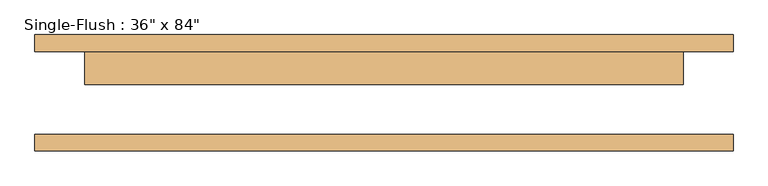
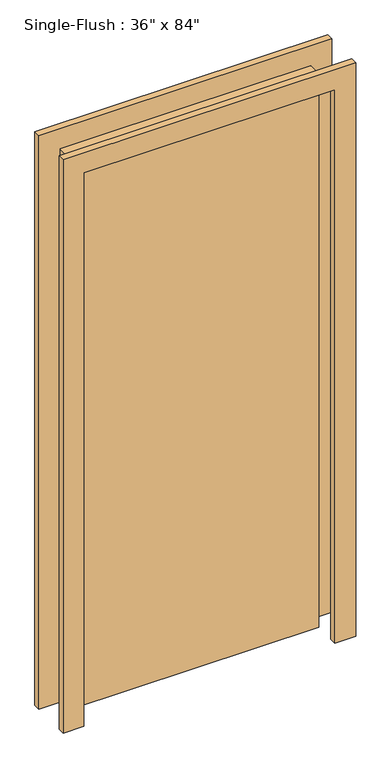
"""IFC4 building model written with IfcOpenShell, lengths in millimetres: door geometry."""

from ifc_helpers import new_model, si_unit, frame, origin, origin_with_axes, place, context, project, spatial, polyline, outline, extrude, source, transform, mapped, element, save


def door_a1797ceb(model_context):
    return source(origin(), model_context, "Body", "SweptSolid", [
        extrude(outline(polyline([(2209.8, -533.4), (0.0, -533.4), (0.0, -457.2), (2133.6, -457.2), (2133.6, 457.2), (0.0, 457.2), (0.0, 533.4), (2209.8, 533.4), (2209.8, -533.4)])), frame((0.0, 63.5, 0.0), z_axis=(0.0, 1.0, 0.0), x_axis=(0.0, 0.0, 1.0)), (0.0, 0.0, 1.0), 25.4),
        extrude(outline(polyline([(2209.8, 533.4), (2209.8, -533.4), (0.0, -533.4), (0.0, -457.2), (2133.6, -457.2), (2133.6, 457.2), (0.0, 457.2), (0.0, 533.4), (2209.8, 533.4)])), frame((0.0, -88.9, 0.0), z_axis=(0.0, 1.0, 0.0), x_axis=(0.0, 0.0, 1.0)), (0.0, 0.0, 1.0), 25.4),
        extrude(outline(polyline([(457.2, 12.7), (-457.2, 12.7), (-457.2, 63.5), (457.2, 63.5), (457.2, 12.7)])), origin_with_axes(), (0.0, 0.0, 1.0), 2133.6),
    ])


if __name__ == "__main__":
    model = new_model("IFC4")
    model_context = context("Model", 3, world=origin())
    ifc_project = project(units=[si_unit("LENGTHUNIT", "METRE", prefix="MILLI")], contexts=[model_context])
    site = spatial("IfcSite", under=ifc_project)
    building = spatial("IfcBuilding", under=site)
    placement = place(None, origin())
    door_shape = door_a1797ceb(model_context)
    element("IfcDoor", 1, ObjectType="Single-Flush : 36\" x 84\"", at=placement, inside=building, context=model_context, shape_type="MappedRepresentation", body=[
        mapped(door_shape, transform((0.0, 0.0, 0.0), x_axis=(1.0, 0.0, 0.0), y_axis=(0.0, 1.0, 0.0), z_axis=(0.0, 0.0, 1.0))),
    ])
    save(model, "model.ifc")

# Revit data of these elements
# Type "Single-Flush : 36\" x 84\""
#   Type Mark = "1"
#   Assembly Code = "C1020"
#   Thickness = 0' - 2"
#   Height = 7' - 0"
#   Trim Projection Ext = 0' - 1"
#   Trim Projection Int = 0' - 1"
#   Trim Width = 0' - 3"
#   Width = 3' - 0"
#   Door Material = Door - Panel
#   Frame Material = Door - Frame
#   Function = (empty or 0)
#   Wall Closure = (empty or 0)
# Element 1 (IfcDoor, "Single-Flush : 36\" x 84\"")
#   Materials on its faces: "Door - Frame", "Door - Panel"
# Materials
#   "Door - Panel": class "Wood", colour RGB 114 82 51, transparency 0
#   "Door - Frame": colour RGB 153 76 43, transparency 0
